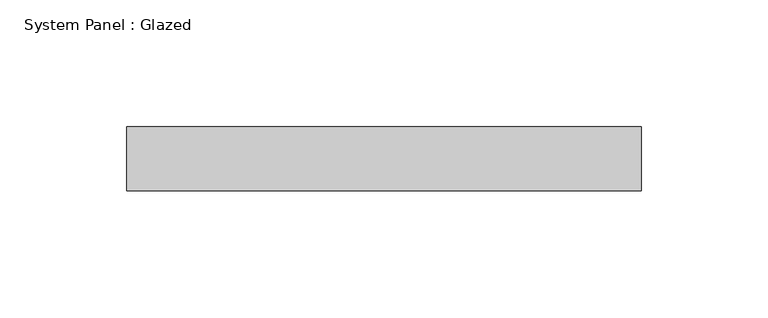
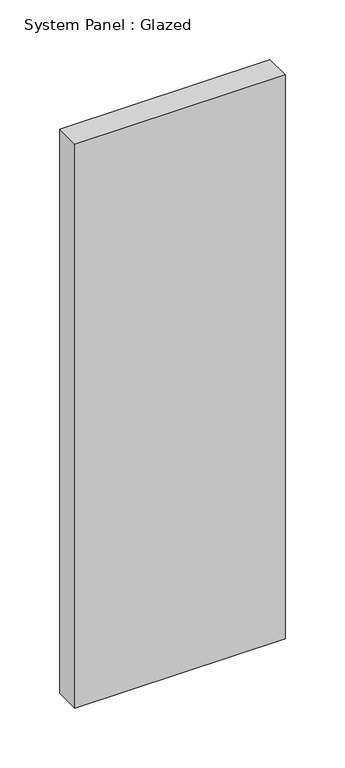
"""IFC4 building model written with IfcOpenShell, lengths in millimetres: plate geometry, System Panel : Glazed."""

from ifc_helpers import new_model, si_unit, origin, origin_with_axes, place, context, project, spatial, polyline, outline, extrude, source, transform, mapped, element, save


def system_panel_glazed_dfb1dee4(model_context):
    return source(origin(), model_context, "Body", "SweptSolid", [
        extrude(outline(polyline([(101.6, 19.05), (-101.6, 19.05), (-101.6, 44.45), (101.6, 44.45), (101.6, 19.05)])), origin_with_axes(), (0.0, 0.0, 1.0), 576.2075706),
    ])


if __name__ == "__main__":
    model = new_model("IFC4")
    model_context = context("Model", 3, world=origin())
    ifc_project = project(units=[si_unit("LENGTHUNIT", "METRE", prefix="MILLI")], contexts=[model_context])
    site = spatial("IfcSite", under=ifc_project)
    building = spatial("IfcBuilding", under=site)
    placement = place(None, origin())
    system_panel_glazed_shape = system_panel_glazed_dfb1dee4(model_context)
    element("IfcPlate", 1, ObjectType="System Panel : Glazed", at=placement, inside=building, context=model_context, shape_type="MappedRepresentation", body=[
        mapped(system_panel_glazed_shape, transform((0.0, 0.0, 0.0), x_axis=(1.0, 0.0, 0.0), y_axis=(0.0, 1.0, 0.0), z_axis=(0.0, 0.0, 1.0))),
    ])
    save(model, "model.ifc")

# Revit data of these elements
# Type "System Panel : Glazed"
#   Construction Type Id = "GSP4R"
#   Analytic Construction = "1/8 in Pilkington single glazing"
#   Visual Light Transmittance = 0.9
#   Solar Heat Gain Coefficient = 0.86
#   Heat Transfer Coefficient (U) = 1.18115 BTU/(h·ft²·°F)
#   Define Thermal Properties by = 1
# Element 1 (IfcPlate, "System Panel : Glazed")
#   Materials on its faces: "Glass"
# Materials
#   "Glass": class "Glass", colour RGB 0 128 192, transparency 0.75, Description = "Soda Lime Glass", Cost = 0
